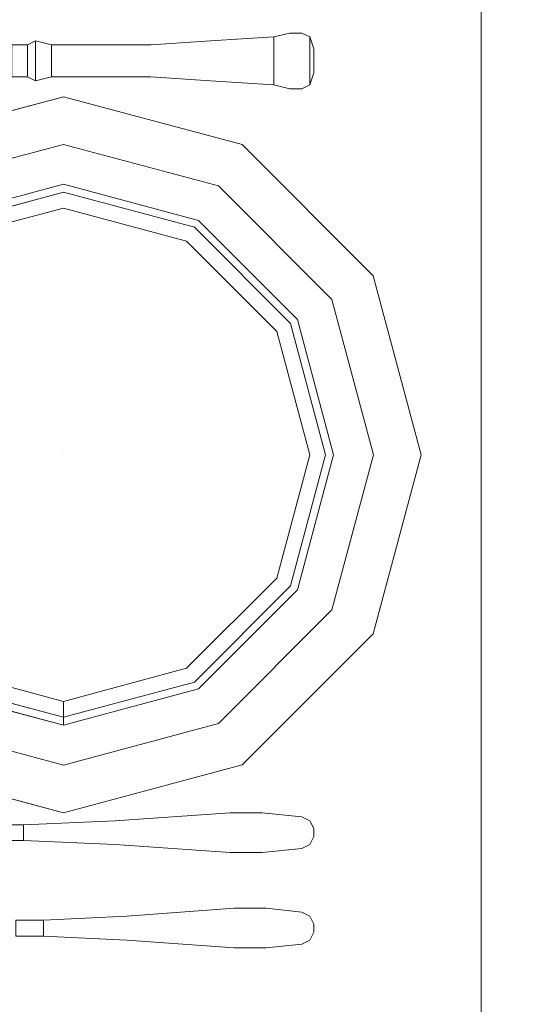
# Model space of a CAD drawing. Units: inches. Extents: x 375 to 1122, y 27 to 1069.
# Tile 145 of 155: x 739.09 to 747.02, y 886.61 to 901.85. Entities that reach past the tile are written whole.
import ezdxf

# ---------------------------------------------------------------- set-up
doc = ezdxf.new("R2010")
doc.units = ezdxf.units.IN
doc.layers.add('A-ANNO-DIMS', color=2, linetype='Continuous', lineweight=18)
doc.layers.add('Furniture', color=30, linetype='Continuous', lineweight=18)
doc.styles.get("Standard").update_dxf_attribs({"font": 'arial.ttf'})
doc.dimstyles.new('ISO-25', dxfattribs={"dimtxt": 12, "dimasz": 2.5, "dimexe": 1.5, "dimexo": 1.5, "dimtad": 1, "dimdec": 1, "dimlunit": 3, "dimtxsty": 'Standard', "dimblk": 'ARCHTICK', "dimcen": 2.5, "dimadec": 0, "dimazin": 0, "dimtfac": 1, "dimtdec": 1, "dimtmove": 0, "dimatfit": 3, "dimfxl": 1.5, "dimfxlon": 1, "dimarcsym": 0})

# ---------------------------------------------------------------- blocks, each defined once
blk = doc.blocks.new('A$C403C54AD')
blk.add_line((0.83575, 1.53256, -0.0006), (1.99923, 1.53256, -0.0006))
at = {"linetype": 'ByBlock'}
for points, invisible_edges in [([(1.0802, 1.50922, -0.02349), (1.0802, 1.49075, -0.02349), (1.02018, 1.47466, -0.02349), (1.01094, 1.49066, -0.02349)], 5), ([(1.0802, 1.47535, -0.03734), (1.0802, 1.50922, -0.02811), (1.01094, 1.49066, -0.02811), (1.02787, 1.46133, -0.03734)], 5), ([(1.14947, 1.49066, -0.02349), (1.14023, 1.47466, -0.02349), (1.0802, 1.49075, -0.02349), (1.0802, 1.50922, -0.02349)], 5), ([(1.13254, 1.46133, -0.03734), (1.14947, 1.49066, -0.02811), (1.0802, 1.50922, -0.02811), (1.0802, 1.47535, -0.03734)], 5), ([(1.01094, 1.49066, -0.02349), (1.02018, 1.47466, -0.02349), (0.97623, 1.43072, -0.02349), (0.96024, 1.43995, -0.02349)], 5), ([(1.02787, 1.46133, -0.03734), (1.01094, 1.49066, -0.02811), (0.96024, 1.43995, -0.02811), (0.98956, 1.42302, -0.03734)], 5), ([(1.0802, 1.49075, -0.02349), (1.0802, 1.47228, -0.02965), (1.02941, 1.45867, -0.02965), (1.02018, 1.47466, -0.02349)], 5), ([(1.14023, 1.47466, -0.02349), (1.131, 1.45867, -0.02965), (1.0802, 1.47228, -0.02965), (1.0802, 1.49075, -0.02349)], 5), ([(1.17085, 1.42302, -0.03734), (1.20017, 1.43995, -0.02811), (1.14947, 1.49066, -0.02811), (1.13254, 1.46133, -0.03734)], 5), ([(1.20017, 1.43995, -0.02349), (1.18418, 1.43072, -0.02349), (1.14023, 1.47466, -0.02349), (1.14947, 1.49066, -0.02349)], 5), ([(1.02018, 1.47466, -0.02349), (1.02941, 1.45867, -0.02965), (0.99223, 1.42148, -0.02965), (0.97623, 1.43072, -0.02349)], 5), ([(1.0802, 1.46612, -0.04658), (1.0802, 1.47535, -0.03734), (1.02787, 1.46133, -0.03734), (1.03249, 1.45333, -0.04658)], 5), ([(1.12792, 1.45333, -0.04658), (1.13254, 1.46133, -0.03734), (1.0802, 1.47535, -0.03734), (1.0802, 1.46612, -0.04658)], 5), ([(1.18418, 1.43072, -0.02349), (1.16818, 1.42148, -0.02965), (1.131, 1.45867, -0.02965), (1.14023, 1.47466, -0.02349)], 5), ([(1.0802, 1.47228, -0.02965), (1.0802, 1.37069, -0.02965), (1.0802, 1.37069, -0.02965), (1.02941, 1.45867, -0.02965)], 5), ([(1.131, 1.45867, -0.02965), (1.0802, 1.37069, -0.02965), (1.0802, 1.37069, -0.02965), (1.0802, 1.47228, -0.02965)], 5), ([(1.03249, 1.45333, -0.04658), (1.02787, 1.46133, -0.03734), (0.98956, 1.42302, -0.03734), (0.99756, 1.4184, -0.04658)], 5), ([(1.16285, 1.4184, -0.04658), (1.17085, 1.42302, -0.03734), (1.13254, 1.46133, -0.03734), (1.12792, 1.45333, -0.04658)], 5), ([(1.02941, 1.45867, -0.02965), (1.0802, 1.37069, -0.02965), (1.0802, 1.37069, -0.02965), (0.99223, 1.42148, -0.02965)], 5), ([(1.16818, 1.42148, -0.02965), (1.0802, 1.37069, -0.02965), (1.0802, 1.37069, -0.02965), (1.131, 1.45867, -0.02965)], 5), ([(0.96024, 1.43995, -0.02349), (0.97623, 1.43072, -0.02349), (0.96015, 1.37069, -0.02349), (0.94168, 1.37069, -0.02349)], 5), ([(0.98956, 1.42302, -0.03734), (0.96024, 1.43995, -0.02811), (0.94168, 1.37069, -0.02811), (0.97554, 1.37069, -0.03734)], 5), ([(1.18487, 1.37069, -0.03734), (1.21873, 1.37069, -0.02811), (1.20017, 1.43995, -0.02811), (1.17085, 1.42302, -0.03734)], 5), ([(1.21873, 1.37069, -0.02349), (1.20026, 1.37069, -0.02349), (1.18418, 1.43072, -0.02349), (1.20017, 1.43995, -0.02349)], 5), ([(0.97623, 1.43072, -0.02349), (0.99223, 1.42148, -0.02965), (0.97862, 1.37069, -0.02965), (0.96015, 1.37069, -0.02349)], 5), ([(1.20026, 1.37069, -0.02349), (1.18179, 1.37069, -0.02965), (1.16818, 1.42148, -0.02965), (1.18418, 1.43072, -0.02349)], 5), ([(0.99756, 1.4184, -0.04658), (0.98956, 1.42302, -0.03734), (0.97554, 1.37069, -0.03734), (0.98477, 1.37069, -0.04658)], 5), ([(0.99223, 1.42148, -0.02965), (1.0802, 1.37069, -0.02965), (1.0802, 1.37069, -0.02965), (0.97862, 1.37069, -0.02965)], 5), ([(1.18179, 1.37069, -0.02965), (1.0802, 1.37069, -0.02965), (1.0802, 1.37069, -0.02965), (1.16818, 1.42148, -0.02965)], 5), ([(1.17563, 1.37069, -0.04658), (1.18487, 1.37069, -0.03734), (1.17085, 1.42302, -0.03734), (1.16285, 1.4184, -0.04658)], 4), ([(0.94168, 1.37069, -0.02349), (0.96015, 1.37069, -0.02349), (0.97623, 1.31066, -0.02349), (0.96024, 1.30143, -0.02349)], 5), ([(0.97554, 1.37069, -0.03734), (0.94168, 1.37069, -0.02811), (0.96024, 1.30143, -0.02811), (0.98956, 1.31836, -0.03734)], 5), ([(0.96015, 1.37069, -0.02349), (0.97862, 1.37069, -0.02965), (0.99223, 1.3199, -0.02965), (0.97623, 1.31066, -0.02349)], 5), ([(0.98477, 1.37069, -0.04658), (0.97554, 1.37069, -0.03734), (0.98956, 1.31836, -0.03734), (0.99756, 1.32297, -0.04658)], 5), ([(0.97862, 1.37069, -0.02965), (1.0802, 1.37069, -0.02965), (1.0802, 1.37069, -0.02965), (0.99223, 1.3199, -0.02965)], 5), ([(0.99223, 1.3199, -0.02965), (1.0802, 1.37069, -0.02965), (1.0802, 1.37069, -0.02965), (1.02941, 1.28271, -0.02965)], 5), ([(1.02941, 1.28271, -0.02965), (1.0802, 1.37069, -0.02965), (1.0802, 1.37069, -0.02965), (1.0802, 1.2691, -0.02965)], 5), ([(1.0802, 1.2691, -0.02965), (1.0802, 1.37069, -0.02965), (1.0802, 1.37069, -0.02965), (1.131, 1.28271, -0.02965)], 5), ([(1.16818, 1.3199, -0.02965), (1.0802, 1.37069, -0.02965), (1.0802, 1.37069, -0.02965), (1.18179, 1.37069, -0.02965)], 5), ([(1.131, 1.28271, -0.02965), (1.0802, 1.37069, -0.02965), (1.0802, 1.37069, -0.02965), (1.16818, 1.3199, -0.02965)], 5), ([(1.18418, 1.31066, -0.02349), (1.16818, 1.3199, -0.02965), (1.18179, 1.37069, -0.02965), (1.20026, 1.37069, -0.02349)], 5), ([(1.17085, 1.31836, -0.03734), (1.20017, 1.30143, -0.02811), (1.21873, 1.37069, -0.02811), (1.18487, 1.37069, -0.03734)], 5), ([(1.20017, 1.30143, -0.02349), (1.18418, 1.31066, -0.02349), (1.20026, 1.37069, -0.02349), (1.21873, 1.37069, -0.02349)], 5)]:
    blk.add_3dface(points, dxfattribs=dict(at, invisible_edges=invisible_edges))
for points in [[(1.0802, 1.50922, -0.02811), (1.0802, 1.50922, -0.02349), (1.01094, 1.49066, -0.02349), (1.01094, 1.49066, -0.02811)], [(1.14947, 1.49066, -0.02811), (1.14947, 1.49066, -0.02349), (1.0802, 1.50922, -0.02349), (1.0802, 1.50922, -0.02811)], [(1.01094, 1.49066, -0.02811), (1.01094, 1.49066, -0.02349), (0.96024, 1.43995, -0.02349), (0.96024, 1.43995, -0.02811)], [(1.20017, 1.43995, -0.02811), (1.20017, 1.43995, -0.02349), (1.14947, 1.49066, -0.02349), (1.14947, 1.49066, -0.02811)], [(0.96024, 1.43995, -0.02811), (0.96024, 1.43995, -0.02349), (0.94168, 1.37069, -0.02349), (0.94168, 1.37069, -0.02811)], [(1.21873, 1.37069, -0.02811), (1.21873, 1.37069, -0.02349), (1.20017, 1.43995, -0.02349), (1.20017, 1.43995, -0.02811)], [(0.94168, 1.37069, -0.02811), (0.94168, 1.37069, -0.02349), (0.96024, 1.30143, -0.02349), (0.96024, 1.30143, -0.02811)], [(1.16285, 1.32297, -0.04658), (1.17085, 1.31836, -0.03734), (1.18487, 1.37069, -0.03734), (1.17563, 1.37069, -0.04658)], [(1.20017, 1.30143, -0.02811), (1.20017, 1.30143, -0.02349), (1.21873, 1.37069, -0.02349), (1.21873, 1.37069, -0.02811)]]:
    blk.add_3dface(points, dxfattribs=at)
for points in [[(0.93706, 1.46612, -0.03734), (0.91859, 1.46612, -0.03734), (0.92321, 1.46766, -0.04042), (0.93244, 1.46766, -0.04042)], [(0.92321, 1.46766, -0.04042), (0.92321, 1.46766, -0.04042), (0.91859, 1.46612, -0.03734), (0.91859, 1.46612, -0.0435)], [(0.93706, 1.46612, -0.0435), (0.91859, 1.46612, -0.0435), (0.92321, 1.46766, -0.04042), (0.93244, 1.46766, -0.04042)], [(0.93706, 1.46612, -0.03734), (0.93706, 1.46612, -0.0435), (0.93244, 1.46766, -0.04042)], [(1.22489, 1.46766, -0.03827), (1.22489, 1.46766, -0.03413), (1.22181, 1.46612, -0.03397), (1.22181, 1.46612, -0.0386)], [(1.22797, 1.46766, -0.03413), (1.22797, 1.46766, -0.03827), (1.22489, 1.46766, -0.03827), (1.22489, 1.46766, -0.03413)], [(1.23105, 1.46612, -0.0386), (1.23105, 1.46612, -0.03397), (1.22797, 1.46766, -0.03413), (1.22797, 1.46766, -0.03827)], [(1.26183, 1.46766, -0.03827), (1.26183, 1.46766, -0.03413), (1.25875, 1.46612, -0.03397), (1.25875, 1.46612, -0.0386)], [(1.26491, 1.46766, -0.03413), (1.26491, 1.46766, -0.03827), (1.26183, 1.46766, -0.03827), (1.26183, 1.46766, -0.03413)], [(1.26799, 1.46612, -0.0386), (1.26799, 1.46612, -0.03397), (1.26491, 1.46766, -0.03413), (1.26491, 1.46766, -0.03827)], [(0.91859, 1.46612, -0.03734), (0.91859, 1.46612, -0.0435), (0.91705, 1.46304, -0.04504), (0.91705, 1.46304, -0.03581)], [(0.91705, 1.46304, -0.03581), (0.91705, 1.46304, -0.04504), (0.91705, 1.45842, -0.04658), (0.91705, 1.45842, -0.03427)], [(0.9386, 1.46304, -0.04504), (0.9386, 1.46304, -0.03581), (0.93706, 1.46612, -0.03734), (0.93706, 1.46612, -0.0435)], [(0.9386, 1.45842, -0.03427), (0.9386, 1.45842, -0.04658), (0.9386, 1.46304, -0.04504), (0.9386, 1.46304, -0.03581)], [(1.22027, 1.46304, -0.03884), (1.22027, 1.46304, -0.03421), (1.21873, 1.44765, -0.03425), (1.21873, 1.44765, -0.03888)], [(1.22181, 1.46612, -0.03397), (1.22181, 1.46612, -0.0386), (1.22027, 1.46304, -0.03884), (1.22027, 1.46304, -0.03421)], [(1.23258, 1.46304, -0.03421), (1.23258, 1.46304, -0.03884), (1.23105, 1.46612, -0.0386), (1.23105, 1.46612, -0.03397)], [(1.23412, 1.44765, -0.03888), (1.23412, 1.44765, -0.03425), (1.23258, 1.46304, -0.03421), (1.23258, 1.46304, -0.03884)], [(1.25721, 1.46304, -0.03884), (1.25721, 1.46304, -0.03421), (1.25567, 1.44919, -0.03425), (1.25567, 1.44919, -0.03888)], [(1.25875, 1.46612, -0.03397), (1.25875, 1.46612, -0.0386), (1.25721, 1.46304, -0.03884), (1.25721, 1.46304, -0.03421)], [(1.26953, 1.46304, -0.03421), (1.26953, 1.46304, -0.03884), (1.26799, 1.46612, -0.0386), (1.26799, 1.46612, -0.03397)], [(1.27106, 1.44919, -0.03888), (1.27106, 1.44919, -0.03425), (1.26953, 1.46304, -0.03421), (1.26953, 1.46304, -0.03884)], [(0.91705, 1.45842, -0.04658), (0.91705, 1.45842, -0.03427), (0.91859, 1.45227, -0.03581), (0.91859, 1.45227, -0.04504)], [(0.93706, 1.45227, -0.04504), (0.93706, 1.45227, -0.03581), (0.9386, 1.45842, -0.03427), (0.9386, 1.45842, -0.04658)], [(0.91859, 1.45227, -0.03581), (0.91859, 1.45227, -0.04504), (0.92013, 1.42764, -0.04658), (0.92013, 1.42764, -0.03427)], [(0.93552, 1.42764, -0.03427), (0.93552, 1.42764, -0.04658), (0.93706, 1.45227, -0.04504), (0.93706, 1.45227, -0.03581)], [(1.21873, 1.44765, -0.03425), (1.21873, 1.44765, -0.03888), (1.21873, 1.43534, -0.03855), (1.21873, 1.43534, -0.03392)], [(1.23412, 1.43534, -0.03392), (1.23412, 1.43534, -0.03855), (1.23412, 1.44765, -0.03888), (1.23412, 1.44765, -0.03425)], [(1.25567, 1.44919, -0.03425), (1.25567, 1.44919, -0.03888), (1.25567, 1.43687, -0.03855), (1.25567, 1.43687, -0.03392)], [(1.27106, 1.43687, -0.03392), (1.27106, 1.43687, -0.03855), (1.27106, 1.44919, -0.03888), (1.27106, 1.44919, -0.03425)], [(0.92013, 1.42764, -0.04658), (0.92013, 1.42764, -0.03427), (0.92167, 1.40455, -0.03427), (0.92167, 1.40455, -0.04658)], [(0.93398, 1.40455, -0.04658), (0.93398, 1.40455, -0.03427), (0.93552, 1.42764, -0.03427), (0.93552, 1.42764, -0.04658)], [(0.92167, 1.40455, -0.03427), (0.92167, 1.40455, -0.04658), (0.92167, 1.36607, -0.04504), (0.92167, 1.36607, -0.03581)], [(0.93398, 1.36607, -0.03581), (0.93398, 1.36607, -0.04504), (0.93398, 1.40455, -0.04658), (0.93398, 1.40455, -0.03427)], [(0.92013, 1.35991, -0.03427), (0.93552, 1.35991, -0.03427), (0.93398, 1.36607, -0.03581), (0.92167, 1.36607, -0.03581)], [(0.92013, 1.35991, -0.04658), (0.93552, 1.35991, -0.04658), (0.93398, 1.36607, -0.04504), (0.92167, 1.36607, -0.04504)], [(0.92167, 1.36607, -0.04504), (0.92167, 1.36607, -0.03581), (0.92013, 1.35991, -0.03427), (0.92013, 1.35991, -0.04658)], [(0.93552, 1.35991, -0.04658), (0.93552, 1.35991, -0.03427), (0.93398, 1.36607, -0.03581), (0.93398, 1.36607, -0.04504)], [(1.26645, 1.36299, -0.02863), (1.26029, 1.36299, -0.02863), (1.26029, 1.35222, -0.03071), (1.26645, 1.35222, -0.03071)], [(1.26645, 1.36299, -0.03122), (1.26029, 1.36299, -0.03122), (1.26029, 1.35222, -0.0333), (1.26645, 1.35222, -0.0333)], [(0.93398, 1.35684, -0.03581), (0.92167, 1.35684, -0.03581), (0.92013, 1.35991, -0.03427), (0.93552, 1.35991, -0.03427)], [(0.93398, 1.35684, -0.04504), (0.92167, 1.35684, -0.04504), (0.92013, 1.35991, -0.04658), (0.93552, 1.35991, -0.04658)], [(0.92013, 1.35991, -0.03427), (0.92013, 1.35991, -0.04658), (0.92167, 1.35684, -0.04504), (0.92167, 1.35684, -0.03581)], [(0.92167, 1.35068, -0.03581), (0.93398, 1.35068, -0.03581), (0.93398, 1.35684, -0.03581), (0.92167, 1.35684, -0.03581)], [(0.92167, 1.35068, -0.04504), (0.93398, 1.35068, -0.04504), (0.93398, 1.35684, -0.04504), (0.92167, 1.35684, -0.04504)], [(0.93398, 1.35684, -0.03581), (0.93398, 1.35684, -0.04504), (0.93552, 1.35991, -0.04658), (0.93552, 1.35991, -0.03427)], [(1.22951, 1.3553, -0.02863), (1.22335, 1.3553, -0.02863), (1.22335, 1.34452, -0.03071), (1.22951, 1.34452, -0.03071)], [(1.22951, 1.3553, -0.03122), (1.22335, 1.3553, -0.03122), (1.22335, 1.34452, -0.0333), (1.22951, 1.34452, -0.0333)]]:
    blk.add_3dface(points)
for points, invisible_edges in [([(1.22797, 1.46766, -0.03413), (1.22489, 1.46766, -0.03413), (1.22181, 1.46612, -0.03397), (1.23105, 1.46612, -0.03397)], 4), ([(1.22797, 1.46766, -0.03827), (1.22489, 1.46766, -0.03827), (1.22181, 1.46612, -0.0386), (1.23105, 1.46612, -0.0386)], 4), ([(1.26491, 1.46766, -0.03413), (1.26183, 1.46766, -0.03413), (1.25875, 1.46612, -0.03397), (1.26799, 1.46612, -0.03397)], 4), ([(1.26491, 1.46766, -0.03827), (1.26183, 1.46766, -0.03827), (1.25875, 1.46612, -0.0386), (1.26799, 1.46612, -0.0386)], 4), ([(0.91705, 1.46304, -0.03581), (0.9386, 1.46304, -0.03581), (0.93706, 1.46612, -0.03734), (0.91859, 1.46612, -0.03734)], 1), ([(0.91705, 1.46304, -0.04504), (0.9386, 1.46304, -0.04504), (0.93706, 1.46612, -0.0435), (0.91859, 1.46612, -0.0435)], 1), ([(0.9386, 1.45842, -0.03427), (0.91705, 1.45842, -0.03427), (0.91705, 1.46304, -0.03581), (0.9386, 1.46304, -0.03581)], 5), ([(0.9386, 1.45842, -0.04658), (0.91705, 1.45842, -0.04658), (0.91705, 1.46304, -0.04504), (0.9386, 1.46304, -0.04504)], 5), ([(1.23258, 1.46304, -0.03421), (1.22027, 1.46304, -0.03421), (1.21873, 1.44765, -0.03425), (1.23412, 1.44765, -0.03425)], 5), ([(1.23258, 1.46304, -0.03884), (1.22027, 1.46304, -0.03884), (1.21873, 1.44765, -0.03888), (1.23412, 1.44765, -0.03888)], 5), ([(1.22181, 1.46612, -0.03397), (1.23105, 1.46612, -0.03397), (1.23258, 1.46304, -0.03421), (1.22027, 1.46304, -0.03421)], 5), ([(1.22181, 1.46612, -0.0386), (1.23105, 1.46612, -0.0386), (1.23258, 1.46304, -0.03884), (1.22027, 1.46304, -0.03884)], 5), ([(1.26953, 1.46304, -0.03421), (1.25721, 1.46304, -0.03421), (1.25567, 1.44919, -0.03425), (1.27106, 1.44919, -0.03425)], 5), ([(1.26953, 1.46304, -0.03884), (1.25721, 1.46304, -0.03884), (1.25567, 1.44919, -0.03888), (1.27106, 1.44919, -0.03888)], 5), ([(1.25875, 1.46612, -0.03397), (1.26799, 1.46612, -0.03397), (1.26953, 1.46304, -0.03421), (1.25721, 1.46304, -0.03421)], 5), ([(1.25875, 1.46612, -0.0386), (1.26799, 1.46612, -0.0386), (1.26953, 1.46304, -0.03884), (1.25721, 1.46304, -0.03884)], 5), ([(0.91859, 1.45227, -0.03581), (0.93706, 1.45227, -0.03581), (0.9386, 1.45842, -0.03427), (0.91705, 1.45842, -0.03427)], 4), ([(0.91859, 1.45227, -0.04504), (0.93706, 1.45227, -0.04504), (0.9386, 1.45842, -0.04658), (0.91705, 1.45842, -0.04658)], 4), ([(0.93552, 1.42764, -0.03427), (0.92013, 1.42764, -0.03427), (0.91859, 1.45227, -0.03581), (0.93706, 1.45227, -0.03581)], 1), ([(0.93552, 1.42764, -0.04658), (0.92013, 1.42764, -0.04658), (0.91859, 1.45227, -0.04504), (0.93706, 1.45227, -0.04504)], 1), ([(1.21873, 1.44765, -0.03425), (1.23412, 1.44765, -0.03425), (1.23412, 1.43534, -0.03392), (1.21873, 1.43534, -0.03392)], 5), ([(1.21873, 1.44765, -0.03888), (1.23412, 1.44765, -0.03888), (1.23412, 1.43534, -0.03855), (1.21873, 1.43534, -0.03855)], 5), ([(1.25567, 1.44919, -0.03425), (1.27106, 1.44919, -0.03425), (1.27106, 1.43687, -0.03392), (1.25567, 1.43687, -0.03392)], 5), ([(1.25567, 1.44919, -0.03888), (1.27106, 1.44919, -0.03888), (1.27106, 1.43687, -0.03855), (1.25567, 1.43687, -0.03855)], 5), ([(1.27106, 1.43687, -0.03392), (1.25567, 1.43687, -0.03392), (1.25875, 1.39532, -0.03153), (1.26799, 1.39532, -0.03153)], 5), ([(1.27106, 1.43687, -0.03855), (1.25567, 1.43687, -0.03855), (1.25875, 1.39532, -0.03461), (1.26799, 1.39532, -0.03461)], 5), ([(1.25567, 1.43687, -0.03855), (1.25567, 1.43687, -0.03392), (1.25875, 1.39532, -0.03153), (1.25875, 1.39532, -0.03461)], 4), ([(1.26799, 1.39532, -0.03461), (1.26799, 1.39532, -0.03153), (1.27106, 1.43687, -0.03392), (1.27106, 1.43687, -0.03855)], 1), ([(1.23412, 1.43534, -0.03392), (1.21873, 1.43534, -0.03392), (1.22181, 1.3907, -0.03153), (1.23105, 1.3907, -0.03153)], 5), ([(1.23412, 1.43534, -0.03855), (1.21873, 1.43534, -0.03855), (1.22181, 1.3907, -0.03461), (1.23105, 1.3907, -0.03461)], 5), ([(1.21873, 1.43534, -0.03855), (1.21873, 1.43534, -0.03392), (1.22181, 1.3907, -0.03153), (1.22181, 1.3907, -0.03461)], 4), ([(1.23105, 1.3907, -0.03461), (1.23105, 1.3907, -0.03153), (1.23412, 1.43534, -0.03392), (1.23412, 1.43534, -0.03855)], 1), ([(0.92167, 1.40455, -0.03427), (0.93398, 1.40455, -0.03427), (0.93552, 1.42764, -0.03427), (0.92013, 1.42764, -0.03427)], 5), ([(0.92167, 1.40455, -0.04658), (0.93398, 1.40455, -0.04658), (0.93552, 1.42764, -0.04658), (0.92013, 1.42764, -0.04658)], 5), ([(0.93398, 1.36607, -0.03581), (0.92167, 1.36607, -0.03581), (0.92167, 1.40455, -0.03427), (0.93398, 1.40455, -0.03427)], 4), ([(0.93398, 1.36607, -0.04504), (0.92167, 1.36607, -0.04504), (0.92167, 1.40455, -0.04658), (0.93398, 1.40455, -0.04658)], 4), ([(1.25875, 1.39532, -0.03153), (1.26799, 1.39532, -0.03153), (1.26645, 1.36299, -0.02863), (1.26029, 1.36299, -0.02863)], 1), ([(1.25875, 1.39532, -0.03153), (1.25875, 1.39532, -0.03461), (1.26029, 1.36299, -0.03122), (1.26029, 1.36299, -0.02863)], 5), ([(1.25875, 1.39532, -0.03461), (1.26799, 1.39532, -0.03461), (1.26645, 1.36299, -0.03122), (1.26029, 1.36299, -0.03122)], 1), ([(1.26645, 1.36299, -0.02863), (1.26645, 1.36299, -0.03122), (1.26799, 1.39532, -0.03461), (1.26799, 1.39532, -0.03153)], 5), ([(1.22181, 1.3907, -0.03153), (1.23105, 1.3907, -0.03153), (1.22951, 1.3553, -0.02863), (1.22335, 1.3553, -0.02863)], 1), ([(1.22181, 1.3907, -0.03153), (1.22181, 1.3907, -0.03461), (1.22335, 1.3553, -0.03122), (1.22335, 1.3553, -0.02863)], 5), ([(1.22181, 1.3907, -0.03461), (1.23105, 1.3907, -0.03461), (1.22951, 1.3553, -0.03122), (1.22335, 1.3553, -0.03122)], 1), ([(1.22951, 1.3553, -0.02863), (1.22951, 1.3553, -0.03122), (1.23105, 1.3907, -0.03461), (1.23105, 1.3907, -0.03153)], 5), ([(1.26029, 1.36299, -0.03122), (1.26029, 1.36299, -0.02863), (1.26029, 1.35222, -0.03071), (1.26029, 1.35222, -0.0333)], 5), ([(1.26645, 1.35222, -0.0333), (1.26645, 1.35222, -0.03071), (1.26645, 1.36299, -0.02863), (1.26645, 1.36299, -0.03122)], 5), ([(0.92167, 1.35684, -0.04504), (0.92167, 1.35684, -0.03581), (0.92167, 1.35068, -0.03581), (0.92167, 1.35068, -0.04504)], 4), ([(0.93398, 1.35068, -0.04504), (0.93398, 1.35068, -0.03581), (0.93398, 1.35684, -0.03581), (0.93398, 1.35684, -0.04504)], 1), ([(1.22335, 1.3553, -0.03122), (1.22335, 1.3553, -0.02863), (1.22335, 1.34452, -0.03071), (1.22335, 1.34452, -0.0333)], 5), ([(1.22951, 1.34452, -0.0333), (1.22951, 1.34452, -0.03071), (1.22951, 1.3553, -0.02863), (1.22951, 1.3553, -0.03122)], 5)]:
    blk.add_3dface(points, dxfattribs=dict(invisible_edges=invisible_edges))
blk = doc.blocks.new('_ArchTick')
at = {"color": 0, "linetype": 'ByBlock', "const_width": 0.15}
blk.add_lwpolyline([(-0.5, -0.5), (0.5, 0.5)], dxfattribs=at)
blk = doc.blocks.new('*D73')
at = {"layer": 'A-ANNO-DIMS', "color": 0, "lineweight": -2, "transparency": 16777216}
for p, q in [((686.757, 932.428), (686.757, 929.428)), ((770.757, 932.428), (770.757, 929.428)), ((686.757, 930.928), (770.757, 930.928)), ((770.757, 930.928), (987.61, 930.928))]:
    blk.add_line(p, q, dxfattribs=at)
at = {"layer": 'Defpoints', "color": 0, "transparency": 16777216}
for p in [(686.757, 943.528), (770.757, 943.528), (770.757, 930.928)]:
    blk.add_point(p, dxfattribs=at)
at = {"layer": 'A-ANNO-DIMS', "color": 0, "lineweight": -2, "transparency": 16777216, "xscale": 2.5, "yscale": 2.5, "zscale": 2.5, "rotation": 180}
blk.add_blockref('_ArchTick', (686.757, 930.928), dxfattribs=at)
at = {"layer": 'A-ANNO-DIMS', "color": 0, "lineweight": -2, "transparency": 16777216, "xscale": 2.5, "yscale": 2.5, "zscale": 2.5}
blk.add_blockref('_ArchTick', (770.757, 930.928), dxfattribs=at)
at = {"layer": 'A-ANNO-DIMS', "color": 0, "transparency": 16777216, "insert": (880.433, 937.757), "char_height": 12, "attachment_point": 5}
blk.add_mtext('2-PANEL SLIDER 7\'-0" TYP.', dxfattribs=at)
blk = doc.blocks.new('*D88')
at = {"layer": 'A-ANNO-DIMS', "color": 0, "lineweight": -2, "transparency": 16777216}
for p, q in [((731.007, 1052.528), (731.007, 1055.528)), ((854.007, 1052.528), (854.007, 1055.528)), ((731.007, 1054.028), (854.007, 1054.028))]:
    blk.add_line(p, q, dxfattribs=at)
at = {"layer": 'Defpoints', "color": 0, "transparency": 16777216}
for p in [(854.007, 1054.028), (731.007, 502.528), (854.007, 502.528)]:
    blk.add_point(p, dxfattribs=at)
at = {"layer": 'A-ANNO-DIMS', "color": 0, "lineweight": -2, "transparency": 16777216, "xscale": 2.5, "yscale": 2.5, "zscale": 2.5, "rotation": 180}
blk.add_blockref('_ArchTick', (731.007, 1054.028), dxfattribs=at)
at = {"layer": 'A-ANNO-DIMS', "color": 0, "lineweight": -2, "transparency": 16777216, "xscale": 2.5, "yscale": 2.5, "zscale": 2.5}
blk.add_blockref('_ArchTick', (854.007, 1054.028), dxfattribs=at)
at = {"layer": 'A-ANNO-DIMS', "color": 0, "transparency": 16777216, "insert": (792.507, 1060.784), "char_height": 12, "attachment_point": 5}
blk.add_mtext('10\'-3"', dxfattribs=at)
blk = doc.blocks.new('*D91')
at = {"layer": 'A-ANNO-DIMS', "color": 0, "lineweight": -2, "transparency": 16777216}
for p, q in [((728.007, 1052.528), (728.007, 1055.528)), ((788.007, 1052.528), (788.007, 1055.528)), ((728.007, 1054.028), (788.007, 1054.028))]:
    blk.add_line(p, q, dxfattribs=at)
at = {"layer": 'Defpoints', "color": 0, "transparency": 16777216}
for p in [(788.007, 1054.028), (728.007, 774.028), (788.007, 774.028)]:
    blk.add_point(p, dxfattribs=at)
at = {"layer": 'A-ANNO-DIMS', "color": 0, "lineweight": -2, "transparency": 16777216, "xscale": 2.5, "yscale": 2.5, "zscale": 2.5, "rotation": 180}
blk.add_blockref('_ArchTick', (728.007, 1054.028), dxfattribs=at)
at = {"layer": 'A-ANNO-DIMS', "color": 0, "lineweight": -2, "transparency": 16777216, "xscale": 2.5, "yscale": 2.5, "zscale": 2.5}
blk.add_blockref('_ArchTick', (788.007, 1054.028), dxfattribs=at)
at = {"layer": 'A-ANNO-DIMS', "color": 0, "transparency": 16777216, "insert": (758.007, 1060.78), "char_height": 12, "attachment_point": 5}
blk.add_mtext('5\'-0"', dxfattribs=at)

msp = doc.modelspace()

# ---------------------------------------------------------------- block references
at = {"layer": 'Furniture', "xscale": 39.9918517141215, "yscale": 39.9918517141215, "zscale": 39.9918517141215, "rotation": 270}
msp.add_blockref('A$C403C54AD', (684.955, 938.316, 0.024), dxfattribs=at)

# ---------------------------------------------------------------- dimensions: what is measured, and where the dimension line sits
at = {"layer": 'A-ANNO-DIMS'}
for base, p1, p2, picture, middle in [((788.007, 1054.028), (728.007, 774.028), (788.007, 774.028), '*D91', (758.007, 1060.78)), ((854.007, 1054.028), (731.007, 502.528), (854.007, 502.528), '*D88', (792.507, 1060.784))]:
    dim = msp.add_linear_dim(base=base, p1=p1, p2=p2, dimstyle='ISO-25', override={"dimdec": 1, "dimlfac": 1, "dimrnd": 0, "dimzin": 1, "dimdsep": 46, "dimlunit": 4, "dimfrac": 2}, dxfattribs=at)
    dim.commit()
    dim.dimension.update_dxf_attribs({"geometry": picture, "text_midpoint": middle})
dim = msp.add_linear_dim(base=(770.757, 930.928), p1=(686.757, 943.528), p2=(770.757, 943.528), text='2-PANEL SLIDER <> TYP.', dimstyle='ISO-25', override={"dimdec": 1, "dimlfac": 1, "dimrnd": 0, "dimzin": 1, "dimdsep": 46, "dimlunit": 4, "dimfrac": 2}, dxfattribs=at)
dim.commit()
dim.dimension.update_dxf_attribs({"geometry": '*D73', "text_midpoint": (880.433, 937.757)})

doc.saveas('drawing.dxf')
